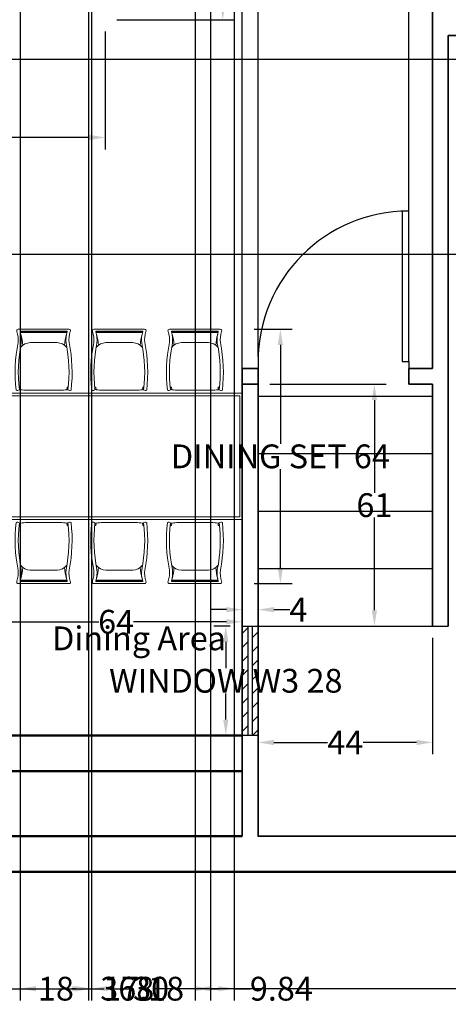
# Model space of a CAD drawing. Units: inches. Extents: x -1285 to -837, y -84 to 552.
# Tile 3 of 10: x -1089 to -981, y -84 to 164. Entities that reach past the tile are written whole.
import ezdxf

# ---------------------------------------------------------------- set-up
doc = ezdxf.new("R2010")
doc.units = ezdxf.units.IN
doc.header["$MEASUREMENT"] = 0
for name, color, linetype, lineweight in [('A-ANNO-DIMS', 2, 'Continuous', 18), ('A-AREA-IDEN', 7, 'Continuous', 25), ('A-GLAZ-PATT', 191, 'Continuous', 13), ('Dining Table', 52, 'Continuous', 18), ('Doors', 34, 'Continuous', 25), ('Inner Wall', 202, 'Continuous', 35), ('Outer Wall', 12, 'Continuous', 50), ('Stairs', 90, 'Continuous', 25), ('Windows', 191, 'Continuous', 25)]:
    doc.layers.add(name, color=color, linetype=linetype, lineweight=lineweight)
doc.styles.get("Standard").update_dxf_attribs({"font": 'arial.ttf'})
doc.dimstyles.get("Standard").update_dxf_attribs({"dimtxt": 6, "dimasz": 4, "dimexe": 3, "dimexo": 3, "dimgap": 0.09, "dimtad": 0, "dimtih": 1, "dimtoh": 1, "dimdec": 1, "dimzin": 0, "dimdsep": 46, "dimlunit": 3, "dimtxsty": 'Standard', "dimcen": 0.09, "dimadec": 0, "dimazin": 0, "dimtfac": 1, "dimtdec": 1, "dimtofl": 0, "dimtmove": 0, "dimatfit": 3, "dimfxl": 1, "dimtolj": 1, "dimtzin": 0, "dimarcsym": 0})

# ---------------------------------------------------------------- blocks, each defined once
blk = doc.blocks.new('A$C51F1')
at = {"color": 0}
for p, q in [((0.2273, 0.4758), (0.0436, 0.4758)), ((0.2273, 0.4758), (0.4111, 0.4758)), ((0.2273, 0.4676), (0.0439, 0.4676)), ((0.2273, 0.4668), (0.0439, 0.4668)), ((0.2273, 0.4676), (0.4107, 0.4676)), ((0.2273, 0.4668), (0.4107, 0.4668)), ((0.2273, 0.3858), (0.1205, 0.3858)), ((0.2273, 0.3858), (0.3341, 0.3858)), ((0.0417, 0.0321), (0.0321, 0.0321)), ((0.0417, 0.0321), (0.0326, 0.0278)), ((0.0435, 0.0127), (0.0417, 0.0321)), ((0.4112, 0.0127), (0.4129, 0.0321)), ((0.4129, 0.0321), (0.4225, 0.0321)), ((0.4129, 0.0321), (0.4221, 0.0278))]:
    blk.add_line(p, q, dxfattribs=at)
blk.add_lwpolyline([(0.4387, 0.4737, 0.102523), (0.4291, 0.3863, -0.080461), (0.4447, 0.0091, -0.3023), (0.4203, 0.012, 0.197932), (0.4111, 0.0127, -0.028193), (0.3571, 0.0091), (0.227, 0.0091), (0.097, 0.0091, -0.028193), (0.0429, 0.0127, 0.197932), (0.0338, 0.012, -0.3023), (0.0093, 0.0091, -0.080461), (0.0249, 0.3863, 0.102523), (0.0153, 0.4737, -0.587111), (0.0261, 0.4929), (0.4279, 0.4929, -0.587111)], format="xyb", close=True, dxfattribs=at)
for centre, radius, start, end in [((0.044, 0.4735), 0.00242, 100.34496, 201.37417), ((-0.1898, 0.4063), 0.2409, 354.55133, 15.96258), ((0.6445, 0.4063), 0.2409, 164.03742, 185.44867), ((0.4106, 0.4735), 0.00242, 338.62583, 79.65504), ((0.0439, 0.4669), 0.000725, 87.37617, 197.52085), ((0.0438, 0.4664), 0.000433, 71.7715, 189.22024), ((-0.2563, 0.3584), 0.3173, 1.15909, 17.56409), ((0.7109, 0.3584), 0.3173, 162.43591, 178.84091), ((0.4107, 0.4669), 0.000725, 342.47915, 92.62383), ((0.4109, 0.4664), 0.000433, 350.77976, 108.2285), ((1.1806, 0.1494), 1.1544, 168.43567, 186.83625), ((0.1214, 0.2879), 0.0978, 90.51639, 143.19267), ((0.3332, 0.2879), 0.0978, 36.80733, 89.48361), ((-0.7259, 0.1494), 1.1544, 353.16375, 11.56433), ((0.0397, 0.0013), 0.012, 71.75361, 116.5375), ((0.4149, 0.0013), 0.012, 63.4625, 108.24639)]:
    blk.add_arc(centre, radius, start, end, dxfattribs=at)
blk = doc.blocks.new('Dining Table')
at = {"color": 0, "ltscale": 0.5}
for points in [[(5887.4, 1648.9), (7887.4, 1648.9), (7887.4, 2648.9), (5887.4, 2648.9)], [(5907.4, 1668.9), (7867.4, 1668.9), (7867.4, 2628.9), (5907.4, 2628.9)]]:
    blk.add_lwpolyline(points, close=True, dxfattribs=at)
at = {"color": 0, "ltscale": 0.5, "yscale": 1000, "zscale": 1000}
for p, xscale in [((6085.4, 2664.8), 1000), ((6685.4, 2664.8), 1000), ((7739.4, 2664.8), -1000)]:
    blk.add_blockref('A$C51F1', p, dxfattribs=dict(at, xscale=xscale))
at = {"color": 0, "ltscale": 0.5, "yscale": 1000, "zscale": 1000, "rotation": 180}
for p, xscale in [((6085.4, 1633), -1000), ((6685.4, 1633), -1000), ((7739.4, 1633), 1000)]:
    blk.add_blockref('A$C51F1', p, dxfattribs=dict(at, xscale=xscale))
blk = doc.blocks.new('*U18')
for p, q in [((-40, 0), (-40, -6)), ((0, 0), (0, -6))]:
    blk.add_line(p, q)
blk.add_lwpolyline([(0, 0), (0, 40), (-1.75, 40), (-1.75, 0)], close=True)
blk.add_arc((0, 0), 40, 90, 180)
blk = doc.blocks.new('Window 1.1')
for p, q in [((1437.47, 769.68), (1441.47, 769.68)), ((1437.47, 742.08), (1437.47, 769.68)), ((1438.97, 742.08), (1438.97, 769.68)), ((1439.95, 769.68), (1439.95, 742.08)), ((1441.47, 769.68), (1441.47, 742.08)), ((1441.47, 742.08), (1437.47, 742.08))]:
    blk.add_line(p, q)
blk = doc.blocks.new('*D57')
at = {"layer": 'A-ANNO-DIMS', "color": 0, "lineweight": -2, "transparency": 16777216}
for p, q in [((-1029.53, 85.84), (-1019.9, 85.84)), ((-1022.9, 81.84), (-1022.9, 56.94)), ((-1022.9, 25.66), (-1022.9, 50.56)), ((-1029.53, 21.66), (-1019.9, 21.66))]:
    blk.add_line(p, q, dxfattribs=at)
at = {"layer": 'A-ANNO-DIMS', "color": 0, "transparency": 16777216}
for points in [[(-1023.57, 81.84), (-1022.24, 81.84), (-1022.9, 85.84)], [(-1023.57, 25.66), (-1022.24, 25.66), (-1022.9, 21.66)]]:
    blk.add_solid(points, dxfattribs=at)
at = {"layer": 'Defpoints', "color": 0, "transparency": 16777216}
for p in [(-1032.53, 85.84), (-1022.9, 85.84), (-1032.53, 21.66)]:
    blk.add_point(p, dxfattribs=at)
at = {"layer": 'A-ANNO-DIMS', "color": 0, "transparency": 16777216, "insert": (-1022.9, 53.75), "char_height": 6, "attachment_point": 5}
blk.add_mtext('\\A1;DINING SET 64', dxfattribs=at)
blk = doc.blocks.new('*D58')
at = {"layer": 'A-ANNO-DIMS', "color": 0, "lineweight": -2, "transparency": 16777216}
for p, q in [((-1096.15, 18.66), (-1096.15, 9.03)), ((-1032.53, 18.66), (-1032.53, 9.03)), ((-1092.15, 12.03), (-1068.73, 12.03)), ((-1036.53, 12.03), (-1059.95, 12.03))]:
    blk.add_line(p, q, dxfattribs=at)
at = {"layer": 'A-ANNO-DIMS', "color": 0, "transparency": 16777216}
for points in [[(-1092.15, 12.7), (-1092.15, 11.36), (-1096.15, 12.03)], [(-1036.53, 12.7), (-1036.53, 11.36), (-1032.53, 12.03)]]:
    blk.add_solid(points, dxfattribs=at)
at = {"layer": 'Defpoints', "color": 0, "transparency": 16777216}
for p in [(-1096.15, 21.66), (-1032.53, 21.66), (-1032.53, 12.03)]:
    blk.add_point(p, dxfattribs=at)
at = {"layer": 'A-ANNO-DIMS', "color": 0, "transparency": 16777216, "insert": (-1064.34, 12.03), "char_height": 6, "attachment_point": 5}
blk.add_mtext('\\A1;64', dxfattribs=at)
blk = doc.blocks.new('*D61')
at = {"layer": 'A-ANNO-DIMS', "color": 0, "lineweight": -2, "transparency": 16777216}
for p, q in [((-1035.53, 10.94), (-1039.67, 10.94)), ((-1036.67, 6.94), (-1036.67, 0.34)), ((-1036.67, -12.66), (-1036.67, -6.06)), ((-1035.53, -16.66), (-1039.67, -16.66))]:
    blk.add_line(p, q, dxfattribs=at)
at = {"layer": 'A-ANNO-DIMS', "color": 0, "transparency": 16777216}
for points in [[(-1037.34, 6.94), (-1036, 6.94), (-1036.67, 10.94)], [(-1037.34, -12.66), (-1036, -12.66), (-1036.67, -16.66)]]:
    blk.add_solid(points, dxfattribs=at)
at = {"layer": 'Defpoints', "color": 0, "transparency": 16777216}
for p in [(-1036.67, 10.94), (-1032.53, 10.94), (-1032.53, -16.66)]:
    blk.add_point(p, dxfattribs=at)
at = {"layer": 'A-ANNO-DIMS', "color": 0, "transparency": 16777216, "insert": (-1036.67, -2.86), "char_height": 6, "attachment_point": 5}
blk.add_mtext('\\A1;WINDOW W3 28', dxfattribs=at)
blk = doc.blocks.new('*D62')
at = {"layer": 'A-ANNO-DIMS', "color": 0, "lineweight": -2, "transparency": 16777216}
for p, q in [((-1032.53, 13.94), (-1032.53, 18.08)), ((-1028.53, 13.94), (-1028.53, 18.08)), ((-1036.53, 15.08), (-1040.53, 15.08)), ((-1024.53, 15.08), (-1020.53, 15.08))]:
    blk.add_line(p, q, dxfattribs=at)
at = {"layer": 'A-ANNO-DIMS', "color": 0, "transparency": 16777216}
for points in [[(-1036.53, 15.75), (-1036.53, 14.41), (-1032.53, 15.08)], [(-1024.53, 15.75), (-1024.53, 14.41), (-1028.53, 15.08)]]:
    blk.add_solid(points, dxfattribs=at)
at = {"layer": 'Defpoints', "color": 0, "transparency": 16777216}
for p in [(-1028.53, 15.08), (-1032.53, 10.94), (-1028.53, 10.94)]:
    blk.add_point(p, dxfattribs=at)
at = {"layer": 'A-ANNO-DIMS', "color": 0, "transparency": 16777216, "insert": (-1018.36, 15.08), "char_height": 6, "attachment_point": 5}
blk.add_mtext('\\A1;4', dxfattribs=at)
blk = doc.blocks.new('*D65')
at = {"layer": 'A-ANNO-DIMS', "color": 0, "lineweight": -2, "transparency": 16777216}
for p, q in [((-1064.13, 361.96), (-1034.42, 361.96)), ((-1037.42, 357.96), (-1037.42, 266.12)), ((-1037.42, 167.9), (-1037.42, 259.73)), ((-1064.13, 163.9), (-1034.42, 163.9))]:
    blk.add_line(p, q, dxfattribs=at)
at = {"layer": 'A-ANNO-DIMS', "color": 0, "transparency": 16777216}
for points in [[(-1038.09, 357.96), (-1036.75, 357.96), (-1037.42, 361.96)], [(-1038.09, 167.9), (-1036.75, 167.9), (-1037.42, 163.9)]]:
    blk.add_solid(points, dxfattribs=at)
at = {"layer": 'Defpoints', "color": 0, "transparency": 16777216}
for p in [(-1067.13, 361.96), (-1037.42, 361.96), (-1067.13, 163.9)]:
    blk.add_point(p, dxfattribs=at)
at = {"layer": 'A-ANNO-DIMS', "color": 0, "transparency": 16777216, "insert": (-1037.42, 262.93), "char_height": 6, "attachment_point": 5}
blk.add_mtext('\\A1;LOUNGE GROUP 198', dxfattribs=at)
blk = doc.blocks.new('*D66')
at = {"layer": 'A-ANNO-DIMS', "color": 0, "lineweight": -2, "transparency": 16777216}
for p, q in [((-1202.09, 160.9), (-1202.09, 131.19)), ((-1067.13, 160.9), (-1067.13, 131.19)), ((-1198.09, 134.19), (-1141.07, 134.19)), ((-1071.13, 134.19), (-1128.15, 134.19))]:
    blk.add_line(p, q, dxfattribs=at)
at = {"layer": 'A-ANNO-DIMS', "color": 0, "transparency": 16777216}
for points in [[(-1198.09, 134.86), (-1198.09, 133.52), (-1202.09, 134.19)], [(-1071.13, 134.86), (-1071.13, 133.52), (-1067.13, 134.19)]]:
    blk.add_solid(points, dxfattribs=at)
at = {"layer": 'Defpoints', "color": 0, "transparency": 16777216}
for p in [(-1202.09, 163.9), (-1067.13, 163.9), (-1067.13, 134.19)]:
    blk.add_point(p, dxfattribs=at)
at = {"layer": 'A-ANNO-DIMS', "color": 0, "transparency": 16777216, "insert": (-1134.61, 134.19), "char_height": 6, "attachment_point": 5}
blk.add_mtext('\\A1;135', dxfattribs=at)
blk = doc.blocks.new('*D69')
at = {"layer": 'A-ANNO-DIMS', "color": 0, "lineweight": -2, "transparency": 16777216}
for p, q in [((-1245.53, -54.06), (-1245.53, -83.53)), ((-877.53, -54.06), (-877.53, -83.53)), ((-1241.53, -80.53), (-1068.25, -80.53)), ((-881.53, -80.53), (-1054.81, -80.53))]:
    blk.add_line(p, q, dxfattribs=at)
at = {"layer": 'A-ANNO-DIMS', "color": 0, "transparency": 16777216}
for points in [[(-1241.53, -79.86), (-1241.53, -81.2), (-1245.53, -80.53)], [(-881.53, -79.86), (-881.53, -81.2), (-877.53, -80.53)]]:
    blk.add_solid(points, dxfattribs=at)
at = {"layer": 'Defpoints', "color": 0, "transparency": 16777216}
for p in [(-1245.53, -51.06), (-877.53, -51.06), (-877.53, -80.53)]:
    blk.add_point(p, dxfattribs=at)
at = {"layer": 'A-ANNO-DIMS', "color": 0, "transparency": 16777216, "insert": (-1061.53, -80.53), "char_height": 6, "attachment_point": 5}
blk.add_mtext('\\A1;368', dxfattribs=at)
blk = doc.blocks.new('*D80')
at = {"layer": 'A-ANNO-DIMS', "color": 0, "lineweight": -2, "transparency": 16777216}
for p, q in [((-1184.53, -13.66), (-1184.53, 551.29)), ((-1032.53, -13.66), (-1032.53, 551.29)), ((-1180.53, 548.29), (-1114.94, 548.29)), ((-1036.53, 548.29), (-1102.12, 548.29))]:
    blk.add_line(p, q, dxfattribs=at)
at = {"layer": 'A-ANNO-DIMS', "color": 0, "transparency": 16777216}
for points in [[(-1180.53, 548.96), (-1180.53, 547.62), (-1184.53, 548.29)], [(-1036.53, 548.96), (-1036.53, 547.62), (-1032.53, 548.29)]]:
    blk.add_solid(points, dxfattribs=at)
at = {"layer": 'Defpoints', "color": 0, "transparency": 16777216}
for p in [(-1032.53, 548.29), (-1184.53, -16.66), (-1032.53, -16.66)]:
    blk.add_point(p, dxfattribs=at)
at = {"layer": 'A-ANNO-DIMS', "color": 0, "transparency": 16777216, "insert": (-1108.53, 548.29), "char_height": 6, "attachment_point": 5}
blk.add_mtext('\\A1;152', dxfattribs=at)
blk = doc.blocks.new('*D82')
at = {"layer": 'A-ANNO-DIMS', "color": 0, "lineweight": -2, "transparency": 16777216}
for p, q in [((-1028.53, 7.94), (-1028.53, -21.41)), ((-984.53, 7.94), (-984.53, -21.41)), ((-1024.53, -18.41), (-1011.03, -18.41)), ((-988.53, -18.41), (-1002.03, -18.41))]:
    blk.add_line(p, q, dxfattribs=at)
at = {"layer": 'A-ANNO-DIMS', "color": 0, "transparency": 16777216}
for points in [[(-1024.53, -17.74), (-1024.53, -19.08), (-1028.53, -18.41)], [(-988.53, -17.74), (-988.53, -19.08), (-984.53, -18.41)]]:
    blk.add_solid(points, dxfattribs=at)
at = {"layer": 'Defpoints', "color": 0, "transparency": 16777216}
for p in [(-1028.53, 10.94), (-984.53, 10.94), (-1028.53, -18.41)]:
    blk.add_point(p, dxfattribs=at)
at = {"layer": 'A-ANNO-DIMS', "color": 0, "transparency": 16777216, "insert": (-1006.53, -18.41), "char_height": 6, "attachment_point": 5}
blk.add_mtext('\\A1;44', dxfattribs=at)
blk = doc.blocks.new('*D87')
at = {"layer": 'A-ANNO-DIMS', "color": 0, "lineweight": -2, "transparency": 16777216}
for p, q in [((-1070.53, 424.94), (-1070.53, -83.53)), ((-1040.53, 424.94), (-1040.53, -83.53)), ((-1066.53, -80.53), (-1059.9, -80.53)), ((-1044.53, -80.53), (-1051.15, -80.53))]:
    blk.add_line(p, q, dxfattribs=at)
at = {"layer": 'A-ANNO-DIMS', "color": 0, "transparency": 16777216}
for points in [[(-1066.53, -79.86), (-1066.53, -81.2), (-1070.53, -80.53)], [(-1044.53, -79.86), (-1044.53, -81.2), (-1040.53, -80.53)]]:
    blk.add_solid(points, dxfattribs=at)
at = {"layer": 'Defpoints', "color": 0, "transparency": 16777216}
for p in [(-1070.53, 427.94), (-1040.53, 427.94), (-1040.53, -80.53)]:
    blk.add_point(p, dxfattribs=at)
at = {"layer": 'A-ANNO-DIMS', "color": 0, "transparency": 16777216, "insert": (-1055.53, -80.53), "char_height": 6, "attachment_point": 5}
blk.add_mtext('\\A1;30', dxfattribs=at)
blk = doc.blocks.new('*D92')
at = {"layer": 'A-ANNO-DIMS', "color": 0, "lineweight": -2, "transparency": 16777216}
for p, q in [((-1113.53, 153.94), (-845.18, 153.94)), ((-848.18, 149.94), (-848.18, 132.48)), ((-848.18, 108.72), (-848.18, 126.18)), ((-1113.53, 104.72), (-845.18, 104.72))]:
    blk.add_line(p, q, dxfattribs=at)
at = {"layer": 'A-ANNO-DIMS', "color": 0, "transparency": 16777216}
for points in [[(-848.85, 149.94), (-847.51, 149.94), (-848.18, 153.94)], [(-848.85, 108.72), (-847.51, 108.72), (-848.18, 104.72)]]:
    blk.add_solid(points, dxfattribs=at)
at = {"layer": 'Defpoints', "color": 0, "transparency": 16777216}
for p in [(-1116.53, 153.94), (-848.18, 153.94), (-1116.53, 104.72)]:
    blk.add_point(p, dxfattribs=at)
at = {"layer": 'A-ANNO-DIMS', "color": 0, "transparency": 16777216, "insert": (-848.18, 129.33), "char_height": 6, "attachment_point": 5}
blk.add_mtext('\\A1;49.22', dxfattribs=at)
blk = doc.blocks.new('*D93')
at = {"layer": 'A-ANNO-DIMS', "color": 0, "lineweight": -2, "transparency": 16777216}
for p, q in [((-1028.53, 78.94), (-1028.53, 551.29)), ((-990.53, 78.94), (-990.53, 551.29)), ((-1024.53, 548.29), (-1013.92, 548.29)), ((-994.53, 548.29), (-1005.14, 548.29))]:
    blk.add_line(p, q, dxfattribs=at)
at = {"layer": 'A-ANNO-DIMS', "color": 0, "transparency": 16777216}
for points in [[(-1024.53, 548.96), (-1024.53, 547.62), (-1028.53, 548.29)], [(-994.53, 548.96), (-994.53, 547.62), (-990.53, 548.29)]]:
    blk.add_solid(points, dxfattribs=at)
at = {"layer": 'Defpoints', "color": 0, "transparency": 16777216}
for p in [(-990.53, 548.29), (-1028.53, 75.94), (-990.53, 75.94)]:
    blk.add_point(p, dxfattribs=at)
at = {"layer": 'A-ANNO-DIMS', "color": 0, "transparency": 16777216, "insert": (-1009.53, 548.29), "char_height": 6, "attachment_point": 5}
blk.add_mtext('\\A1;38', dxfattribs=at)
blk = doc.blocks.new('*D103')
at = {"layer": 'A-ANNO-DIMS', "color": 0, "lineweight": -2, "transparency": 16777216}
for p, q in [((-1088.53, 506.94), (-1088.53, -83.53)), ((-1071.35, 506.94), (-1071.35, -83.53)), ((-1084.53, -80.53), (-1075.35, -80.53)), ((-1071.35, -80.53), (-1067.35, -80.53))]:
    blk.add_line(p, q, dxfattribs=at)
at = {"layer": 'A-ANNO-DIMS', "color": 0, "transparency": 16777216}
for points in [[(-1084.53, -79.86), (-1084.53, -81.2), (-1088.53, -80.53)], [(-1075.35, -79.86), (-1075.35, -81.2), (-1071.35, -80.53)]]:
    blk.add_solid(points, dxfattribs=at)
at = {"layer": 'Defpoints', "color": 0, "transparency": 16777216}
for p in [(-1088.53, 509.94), (-1071.35, 509.94), (-1071.35, -80.53)]:
    blk.add_point(p, dxfattribs=at)
at = {"layer": 'A-ANNO-DIMS', "color": 0, "transparency": 16777216, "insert": (-1057.41, -80.53), "char_height": 6, "attachment_point": 5}
blk.add_mtext('\\A1;17.18', dxfattribs=at)
blk = doc.blocks.new('*D104')
at = {"layer": 'A-ANNO-DIMS', "color": 0, "lineweight": -2, "transparency": 16777216}
for p, q in [((-1044.37, 506.94), (-1044.37, -83.53)), ((-1034.53, 506.94), (-1034.53, -83.53)), ((-1040.37, -80.53), (-1038.53, -80.53)), ((-1034.53, -80.53), (-1030.53, -80.53))]:
    blk.add_line(p, q, dxfattribs=at)
at = {"layer": 'A-ANNO-DIMS', "color": 0, "transparency": 16777216}
for points in [[(-1040.37, -79.86), (-1040.37, -81.2), (-1044.37, -80.53)], [(-1038.53, -79.86), (-1038.53, -81.2), (-1034.53, -80.53)]]:
    blk.add_solid(points, dxfattribs=at)
at = {"layer": 'Defpoints', "color": 0, "transparency": 16777216}
for p in [(-1044.37, 509.94), (-1034.53, 509.94), (-1034.53, -80.53)]:
    blk.add_point(p, dxfattribs=at)
at = {"layer": 'A-ANNO-DIMS', "color": 0, "transparency": 16777216, "insert": (-1022.66, -80.53), "char_height": 6, "attachment_point": 5}
blk.add_mtext('\\A1;9.84', dxfattribs=at)
blk = doc.blocks.new('*D105')
at = {"layer": 'A-ANNO-DIMS', "color": 0, "lineweight": -2, "transparency": 16777216}
for p, q in [((-1088.53, 428.94), (-1088.53, -83.53)), ((-1070.53, 428.94), (-1070.53, -83.53)), ((-1084.53, -80.53), (-1083.64, -80.53)), ((-1074.53, -80.53), (-1075.42, -80.53))]:
    blk.add_line(p, q, dxfattribs=at)
at = {"layer": 'A-ANNO-DIMS', "color": 0, "transparency": 16777216}
for points in [[(-1084.53, -79.86), (-1084.53, -81.2), (-1088.53, -80.53)], [(-1074.53, -79.86), (-1074.53, -81.2), (-1070.53, -80.53)]]:
    blk.add_solid(points, dxfattribs=at)
at = {"layer": 'Defpoints', "color": 0, "transparency": 16777216}
for p in [(-1088.53, 431.94), (-1070.53, 431.94), (-1070.53, -80.53)]:
    blk.add_point(p, dxfattribs=at)
at = {"layer": 'A-ANNO-DIMS', "color": 0, "transparency": 16777216, "insert": (-1079.53, -80.53), "char_height": 6, "attachment_point": 5}
blk.add_mtext('\\A1;18', dxfattribs=at)
blk = doc.blocks.new('*D121')
at = {"layer": 'A-ANNO-DIMS', "color": 0, "lineweight": -2, "transparency": 16777216}
for p, q in [((-1025.53, 71.94), (-996.18, 71.94)), ((-999.18, 67.94), (-999.18, 44.59)), ((-999.18, 14.94), (-999.18, 38.29)), ((-1025.53, 10.94), (-996.18, 10.94))]:
    blk.add_line(p, q, dxfattribs=at)
at = {"layer": 'A-ANNO-DIMS', "color": 0, "transparency": 16777216}
for points in [[(-999.85, 67.94), (-998.51, 67.94), (-999.18, 71.94)], [(-999.85, 14.94), (-998.51, 14.94), (-999.18, 10.94)]]:
    blk.add_solid(points, dxfattribs=at)
at = {"layer": 'Defpoints', "color": 0, "transparency": 16777216}
for p in [(-1028.53, 71.94), (-1028.53, 10.94), (-999.18, 10.94)]:
    blk.add_point(p, dxfattribs=at)
at = {"layer": 'A-ANNO-DIMS', "color": 0, "transparency": 16777216, "insert": (-999.18, 41.44), "char_height": 6, "attachment_point": 5}
blk.add_mtext('\\A1;61', dxfattribs=at)

msp = doc.modelspace()

# ---------------------------------------------------------------- hatches: boundary and pattern name
at = {"layer": 'A-GLAZ-PATT'}
h = msp.add_hatch(dxfattribs=at)
h.set_pattern_fill('ANSI31', color=256, scale=20)
h.set_pattern_definition([(45, (-2215.271, -696.3812), (-1.767767, 1.767767), [])])
h.paths.add_polyline_path([(-1032.5299, -16.6608), (-1031.0256, -16.6608), (-1031.0256, 10.9392), (-1032.5299, 10.9392)])
h.paths.add_polyline_path([(-1028.5299, 10.9392), (-1030.0527, 10.9392), (-1030.0527, -16.6608), (-1028.5299, -16.6608)])

# ---------------------------------------------------------------- linework, layer by layer
at = {"layer": 'Inner Wall'}
for p, q in [((-984.5299, 180.3238), (-984.5299, 75.9392)), ((-980.5299, 159.9392), (-886.5299, 159.9392)), ((-980.5299, 159.9392), (-980.5299, 10.9392)), ((-1032.5299, 75.9392), (-1032.5299, -42.0608)), ((-1032.5299, 75.9392), (-1028.5299, 75.9392)), ((-990.5299, 75.9392), (-990.5299, 71.9392)), ((-990.5299, 75.9392), (-984.5299, 75.9392)), ((-1032.5299, 71.9392), (-1028.5299, 71.9392)), ((-990.5299, 71.9392), (-984.5299, 71.9392)), ((-984.5299, 71.9392), (-984.5299, 10.9392))]:
    msp.add_line(p, q, dxfattribs=at)
msp.add_lwpolyline([(-1028.5299, 75.9392), (-1028.5299, -42.0608), (-968.24, -42.0608)], dxfattribs=at)
at = {"layer": 'Outer Wall'}
for p, q in [((-1184.5299, -16.6608), (-1032.5299, -16.6608)), ((-1184.5299, -25.6608), (-1032.5299, -25.6608)), ((-1184.5299, -42.0608), (-1032.5299, -42.0608)), ((-1245.5299, -51.0608), (-968.24, -51.0608))]:
    msp.add_line(p, q, dxfattribs=at)
at = {"layer": 'Stairs'}
for p, q in [((-1028.5299, 68.9392), (-984.5299, 68.9392)), ((-1028.5299, 54.4392), (-984.5299, 54.4392)), ((-1028.5299, 39.9392), (-984.5299, 39.9392)), ((-1028.5299, 25.4392), (-984.5299, 25.4392)), ((-1028.5299, 10.9392), (-980.5299, 10.9392))]:
    msp.add_line(p, q, dxfattribs=at)

# ---------------------------------------------------------------- block references
at = {"layer": 'Dining Table', "xscale": 0.0318116679632498, "yscale": 0.0318116679632498, "zscale": 0.0318116679632498}
msp.add_blockref('Dining Table', (-1283.4424, -14.6094), dxfattribs=at)
at = {"layer": 'Doors', "xscale": 0.9500000000000003, "yscale": 0.9500000000000003, "zscale": 0.9500000000000003}
msp.add_blockref('*U18', (-990.5299, 77.6392), dxfattribs=at)
at = {"layer": 'Windows'}
msp.add_blockref('Window 1.1', (-2470.0006, -758.7376), dxfattribs=at)

# ---------------------------------------------------------------- texts
at = {"layer": 'A-AREA-IDEN', "insert": (-1105.4179, 10.8378), "char_height": 6, "attachment_point": 1}
msp.add_mtext_dynamic_manual_height_columns('\\pxqr;Dining Area', width=68.784729, gutter_width=1, heights=[0], dxfattribs=at)

# ---------------------------------------------------------------- dimensions: what is measured, and where the dimension line sits
at = {"layer": 'A-ANNO-DIMS'}
for base, p1, p2, override, picture, middle in [((-1032.5299, 548.2892), (-1184.5299, -16.6608), (-1032.5299, -16.6608), {"dimdec": 0, "dimlfac": 1, "dimrnd": 0, "dimzin": 0, "dimdsep": 46, "dimlunit": 2}, '*D80', (-1108.5299, 548.2892)), ((-990.5299, 548.2892), (-1028.5299, 75.9392), (-990.5299, 75.9392), {"dimdec": 0, "dimlfac": 1, "dimrnd": 0, "dimzin": 0, "dimdsep": 46, "dimlunit": 2}, '*D93', (-1009.5299, 548.2892)), ((-1071.3483, -80.5308), (-1088.5299, 509.9392), (-1071.3483, 509.9392), {"dimdec": 2, "dimlfac": 1, "dimrnd": 0, "dimzin": 0, "dimdsep": 46, "dimlunit": 2}, '*D103', (-1057.4111, -80.5308)), ((-1034.5299, -80.5308), (-1044.3703, 509.9392), (-1034.5299, 509.9392), {"dimdec": 2, "dimlfac": 1, "dimrnd": 0, "dimzin": 0, "dimdsep": 46, "dimlunit": 2}, '*D104', (-1022.6595, -80.5308)), ((-1070.5299, -80.5308), (-1088.5299, 431.9392), (-1070.5299, 431.9392), {"dimdec": 0, "dimlfac": 1, "dimrnd": 0, "dimzin": 0, "dimdsep": 46, "dimlunit": 2}, '*D105', (-1079.5299, -80.5308)), ((-1040.5299, -80.5308), (-1070.5299, 427.9392), (-1040.5299, 427.9392), {"dimdec": 0, "dimlfac": 1, "dimrnd": 0, "dimzin": 0, "dimdsep": 46, "dimlunit": 2}, '*D87', (-1055.5299, -80.5308)), ((-1067.1282, 134.1884), (-1202.088, 163.8976), (-1067.1282, 163.8976), {"dimdec": 0, "dimlfac": 1, "dimrnd": 0, "dimzin": 0, "dimdsep": 46, "dimlunit": 2}, '*D66', (-1134.6081, 134.1884)), ((-1032.5299, 12.0299), (-1096.1532, 21.6576), (-1032.5299, 21.6576), {"dimdec": 0, "dimlfac": 1, "dimrnd": 0, "dimzin": 0, "dimdsep": 46, "dimlunit": 2}, '*D58', (-1064.3415, 12.0299)), ((-1028.5299, 15.0792), (-1032.5299, 10.9392), (-1028.5299, 10.9392), {"dimdec": 0, "dimlfac": 1, "dimrnd": 0, "dimzin": 0, "dimdsep": 46, "dimlunit": 2}, '*D62', (-1018.3648, 15.0792)), ((-877.5299, -80.5308), (-1245.5299, -51.0608), (-877.5299, -51.0608), {"dimdec": 0, "dimlfac": 1, "dimrnd": 0, "dimzin": 0, "dimdsep": 46, "dimlunit": 2}, '*D69', (-1061.5299, -80.5308))]:
    dim = msp.add_linear_dim(base=base, p1=p1, p2=p2, dimstyle='Standard', override=override, dxfattribs=at)
    dim.commit()
    dim.dimension.update_dxf_attribs({"geometry": picture, "text_midpoint": middle})
for base, p1, p2, text, picture, middle in [((-1037.4189, 361.9592), (-1067.1282, 163.8976), (-1067.1282, 361.9592), 'LOUNGE GROUP <>', '*D65', (-1037.4189, 262.9284)), ((-1022.9023, 85.8416), (-1032.5299, 21.6576), (-1032.5299, 85.8416), 'DINING SET <>', '*D57', (-1022.9023, 53.7496)), ((-1036.6699, 10.9392), (-1032.5299, -16.6608), (-1032.5299, 10.9392), 'WINDOW W3 <>', '*D61', (-1036.6699, -2.8608))]:
    dim = msp.add_linear_dim(base=base, p1=p1, p2=p2, angle=90, text=text, dimstyle='Standard', override={"dimdec": 0, "dimlfac": 1, "dimrnd": 0, "dimzin": 0, "dimdsep": 46, "dimlunit": 2}, dxfattribs=at)
    dim.commit()
    dim.dimension.update_dxf_attribs({"geometry": picture, "text_midpoint": middle})
for base, p1, p2, angle, override, picture, middle in [((-848.1799, 153.9392), (-1116.5299, 104.7212), (-1116.5299, 153.9392), 90, {"dimdec": 2, "dimlfac": 1, "dimrnd": 0, "dimzin": 0, "dimdsep": 46, "dimlunit": 2}, '*D92', (-848.1799, 129.3302)), ((-999.1799, 10.9392), (-1028.5299, 71.9392), (-1028.5299, 10.9392), 270, {"dimdec": 0, "dimlfac": 1, "dimrnd": 0, "dimzin": 0, "dimdsep": 46, "dimlunit": 2}, '*D121', (-999.1799, 41.4392)), ((-1028.5299, -18.4108), (-984.5299, 10.9392), (-1028.5299, 10.9392), 180, {"dimdec": 0, "dimlfac": 1, "dimrnd": 0, "dimzin": 0, "dimdsep": 46, "dimlunit": 2}, '*D82', (-1006.5299, -18.4108))]:
    dim = msp.add_linear_dim(base=base, p1=p1, p2=p2, angle=angle, dimstyle='Standard', override=override, dxfattribs=at)
    dim.commit()
    dim.dimension.update_dxf_attribs({"geometry": picture, "text_midpoint": middle})

doc.saveas('drawing.dxf')
